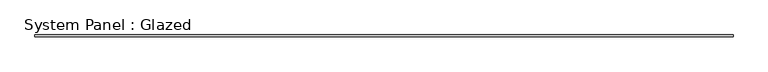
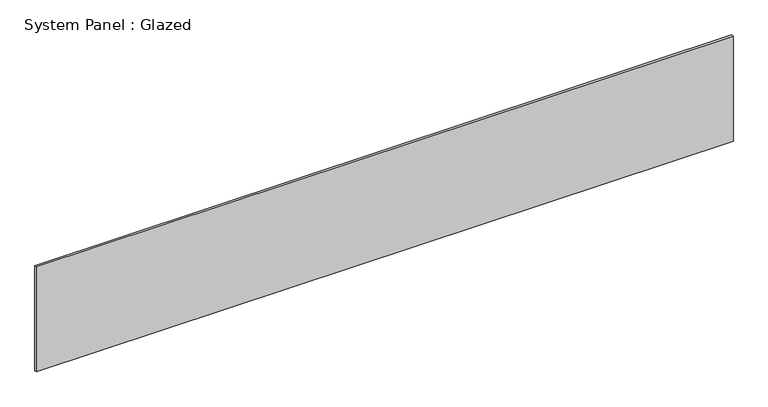
"""IFC4 building model written with IfcOpenShell, lengths in millimetres: plate geometry, System Panel : Glazed."""

from ifc_helpers import new_model, si_unit, origin, origin_with_axes, place, context, project, spatial, polyline, outline, extrude, source, transform, mapped, element, save


def system_panel_glazed_fce9463a(model_context):
    return source(origin(), model_context, "Body", "SweptSolid", [
        extrude(outline(polyline([(4584.7, 19.05), (-4584.7, 19.05), (-4584.7, 44.45), (4584.7, 44.45), (4584.7, 19.05)])), origin_with_axes(), (0.0, 0.0, 1.0), 1460.5),
    ])


if __name__ == "__main__":
    model = new_model("IFC4")
    model_context = context("Model", 3, world=origin())
    ifc_project = project(units=[si_unit("LENGTHUNIT", "METRE", prefix="MILLI")], contexts=[model_context])
    site = spatial("IfcSite", under=ifc_project)
    building = spatial("IfcBuilding", under=site)
    placement = place(None, origin())
    system_panel_glazed_shape = system_panel_glazed_fce9463a(model_context)
    element("IfcPlate", 1, ObjectType="System Panel : Glazed", at=placement, inside=building, context=model_context, shape_type="MappedRepresentation", body=[
        mapped(system_panel_glazed_shape, transform((0.0, 0.0, 0.0), x_axis=(1.0, 0.0, 0.0), y_axis=(0.0, 1.0, 0.0), z_axis=(0.0, 0.0, 1.0))),
    ])
    save(model, "model.ifc")

# Revit data of these elements
# Type "System Panel : Glazed"
#   Construction Type Id = "GSP4R"
#   Analytic Construction = "1/8 in Pilkington single glazing"
#   Visual Light Transmittance = 0.9
#   Solar Heat Gain Coefficient = 0.86
#   Heat Transfer Coefficient (U) = 1.18115 BTU/(h·ft²·°F)
# Element 1 (IfcPlate, "System Panel : Glazed")
#   Materials on its faces: "Glass"
# Materials
#   "Glass": class "Glass", colour RGB 0 128 192, transparency 0.75, Description = "Soda Lime Glass", Cost = 0
